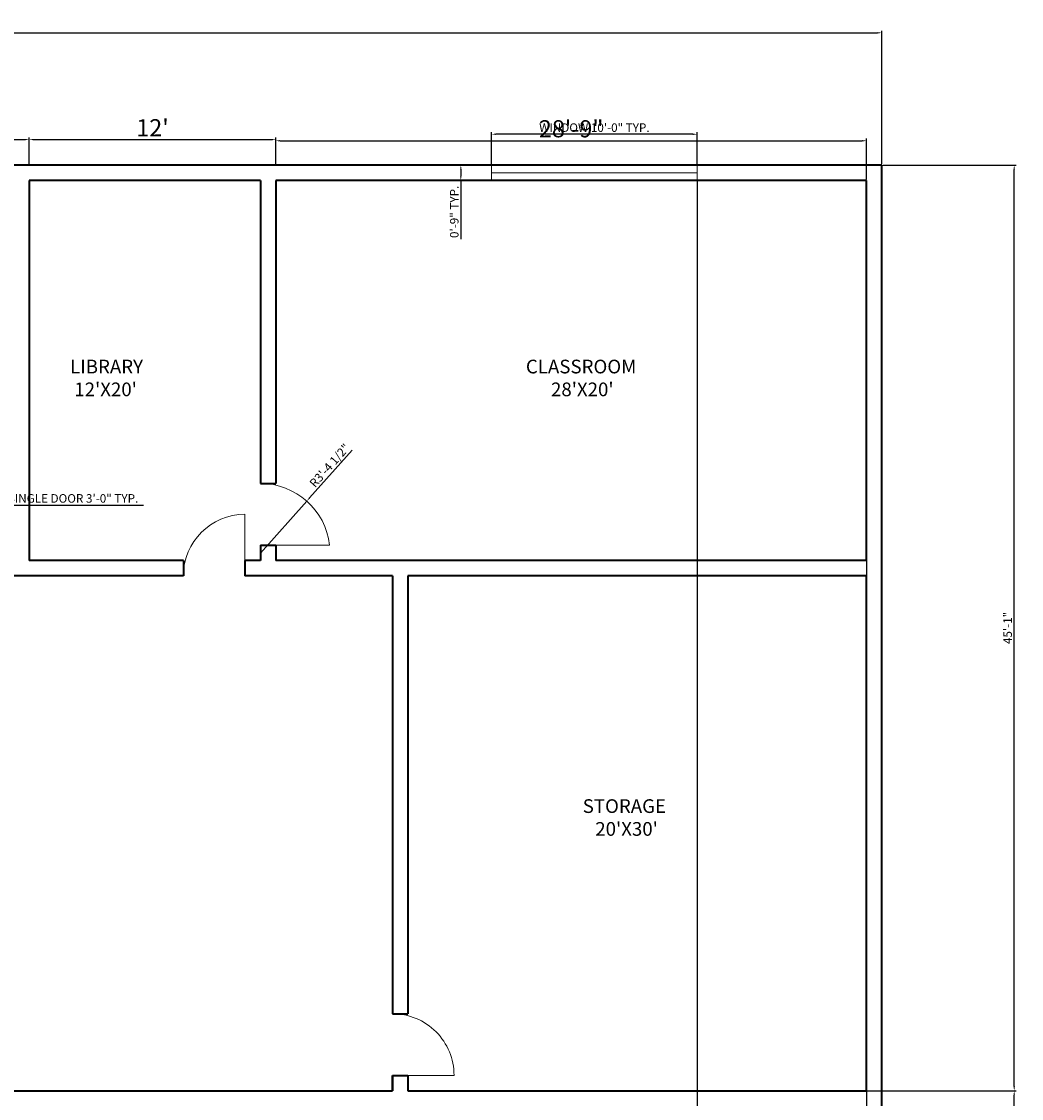
# Model space of a CAD drawing. Units: inches. Extents: x 2394 to 4066, y 1878 to 3193.
# Tile 3 of 3: x 3482 to 4066, y 2560 to 3189. Entities that reach past the tile are written whole.
import ezdxf

# ---------------------------------------------------------------- set-up
doc = ezdxf.new("R2010")
doc.units = ezdxf.units.IN
for name, color, linetype, lineweight in [('A-ANNO-DIMS', 2, 'Continuous', 13), ('A-AREA-IDEN', 7, 'Continuous', 18), ('A-DOOR', 3, 'Continuous', 18), ('A-GLAZ', 4, 'Continuous', 18), ('A-WALL', 7, 'Continuous', 35)]:
    doc.layers.add(name, color=color, linetype=linetype, lineweight=lineweight)
doc.styles.get("Standard").update_dxf_attribs({"font": 'arial.ttf'})
doc.dimstyles.new('ISO-25', dxfattribs={"dimtxt": 5, "dimasz": 2.5, "dimexe": 1.25, "dimexo": 0.625, "dimtad": 1, "dimlunit": 3, "dimtxsty": 'Standard', "dimcen": 2.5, "dimadec": 0, "dimazin": 0, "dimtfac": 1, "dimtmove": 0, "dimatfit": 3, "dimfxl": 1, "dimarcsym": 0})

# ---------------------------------------------------------------- blocks, each defined once
blk = doc.blocks.new('*D3')
at = {"layer": 'A-ANNO-DIMS', "color": 0, "lineweight": -2, "transparency": 16777216}
for p, q in [((3150.1, 3105.72), (3150.1, 3121.22)), ((3486.1, 3105.72), (3486.1, 3121.22)), ((3152.6, 3119.97), (3483.6, 3119.97))]:
    blk.add_line(p, q, dxfattribs=at)
at = {"layer": 'A-ANNO-DIMS', "color": 0, "transparency": 16777216}
for points in [[(3152.6, 3120.39), (3152.6, 3119.56), (3150.1, 3119.97)], [(3483.6, 3120.39), (3483.6, 3119.56), (3486.1, 3119.97)]]:
    blk.add_solid(points, dxfattribs=at)
at = {"layer": 'Defpoints', "color": 0, "transparency": 16777216}
for p in [(3486.1, 3119.97), (3150.1, 3105.09), (3486.1, 3105.09)]:
    blk.add_point(p, dxfattribs=at)
at = {"layer": 'A-ANNO-DIMS', "color": 0, "transparency": 16777216, "insert": (3318.1, 3125.7), "char_height": 10, "attachment_point": 5}
blk.add_mtext("28'", dxfattribs=at)
blk = doc.blocks.new('*D4')
at = {"layer": 'A-ANNO-DIMS', "color": 0, "lineweight": -2, "transparency": 16777216}
for p, q in [((3486.1, 3105.72), (3486.1, 3121.19)), ((3630.1, 3105.72), (3630.1, 3121.19)), ((3488.6, 3119.94), (3627.6, 3119.94))]:
    blk.add_line(p, q, dxfattribs=at)
at = {"layer": 'A-ANNO-DIMS', "color": 0, "transparency": 16777216}
for points in [[(3488.6, 3120.36), (3488.6, 3119.53), (3486.1, 3119.94)], [(3627.6, 3120.36), (3627.6, 3119.53), (3630.1, 3119.94)]]:
    blk.add_solid(points, dxfattribs=at)
at = {"layer": 'Defpoints', "color": 0, "transparency": 16777216}
for p in [(3630.1, 3119.94), (3486.1, 3105.09), (3630.1, 3105.09)]:
    blk.add_point(p, dxfattribs=at)
at = {"layer": 'A-ANNO-DIMS', "color": 0, "transparency": 16777216, "insert": (3558.1, 3125.59), "char_height": 10, "attachment_point": 5}
blk.add_mtext("12'", dxfattribs=at)
blk = doc.blocks.new('*D5')
at = {"layer": 'A-ANNO-DIMS', "color": 0, "lineweight": -2, "transparency": 16777216}
for p, q in [((3630.1, 3105.72), (3630.1, 3120.52)), ((3975.1, 3096.72), (3975.1, 3120.52)), ((3632.6, 3119.27), (3972.6, 3119.27))]:
    blk.add_line(p, q, dxfattribs=at)
at = {"layer": 'A-ANNO-DIMS', "color": 0, "transparency": 16777216}
for points in [[(3632.6, 3119.69), (3632.6, 3118.85), (3630.1, 3119.27)], [(3972.6, 3119.69), (3972.6, 3118.85), (3975.1, 3119.27)]]:
    blk.add_solid(points, dxfattribs=at)
at = {"layer": 'Defpoints', "color": 0, "transparency": 16777216}
for p in [(3975.1, 3119.27), (3630.1, 3105.09), (3975.1, 3096.09)]:
    blk.add_point(p, dxfattribs=at)
at = {"layer": 'A-ANNO-DIMS', "color": 0, "transparency": 16777216, "insert": (3802.6, 3125), "char_height": 10, "attachment_point": 5}
blk.add_mtext('28\'-9"', dxfattribs=at)
blk = doc.blocks.new('DOOR-SINGLE-36IN')
blk.add_line((36, 0), (36, 36))
blk.add_arc((36, 0), 36, 90, 180)
blk = doc.blocks.new('WINDOW-120IN')
for p, q in [((0, 0), (0, 9)), ((120, 0), (120, 9)), ((120, 4.5), (0, 4.5))]:
    blk.add_line(p, q)
blk = doc.blocks.new('*D15')
at = {"layer": 'A-ANNO-DIMS', "color": 0, "lineweight": -2, "transparency": 16777216}
for p, q in [((3432.1, 2901.72), (3432.1, 2907.74)), ((3434.6, 2906.49), (3465.6, 2906.49)), ((3468.1, 2901.72), (3468.1, 2907.74)), ((3468.1, 2906.49), (3552.76, 2906.49))]:
    blk.add_line(p, q, dxfattribs=at)
at = {"layer": 'A-ANNO-DIMS', "color": 0, "transparency": 16777216}
for points in [[(3434.6, 2906.91), (3434.6, 2906.08), (3432.1, 2906.49)], [(3465.6, 2906.91), (3465.6, 2906.08), (3468.1, 2906.49)]]:
    blk.add_solid(points, dxfattribs=at)
at = {"layer": 'Defpoints', "color": 0, "transparency": 16777216}
for p in [(3468.1, 2906.49), (3432.1, 2901.09), (3468.1, 2901.09)]:
    blk.add_point(p, dxfattribs=at)
at = {"layer": 'A-ANNO-DIMS', "color": 0, "transparency": 16777216, "insert": (3511.68, 2909.71), "char_height": 5, "attachment_point": 5}
blk.add_mtext('SINGLE DOOR 3\'-0" TYP.', dxfattribs=at)
blk = doc.blocks.new('*D17')
at = {"layer": 'A-ANNO-DIMS', "color": 0, "lineweight": -2, "transparency": 16777216}
for p, q in [((3756.16, 3105.72), (3756.16, 3124.34)), ((3873.66, 3123.09), (3758.66, 3123.09)), ((3876.16, 3105.72), (3876.16, 3124.34))]:
    blk.add_line(p, q, dxfattribs=at)
at = {"layer": 'A-ANNO-DIMS', "color": 0, "transparency": 16777216}
for points in [[(3758.66, 3123.51), (3758.66, 3122.68), (3756.16, 3123.09)], [(3873.66, 3123.51), (3873.66, 3122.68), (3876.16, 3123.09)]]:
    blk.add_solid(points, dxfattribs=at)
at = {"layer": 'Defpoints', "color": 0, "transparency": 16777216}
for p in [(3756.16, 3123.09), (3756.16, 3105.09), (3876.16, 3105.09)]:
    blk.add_point(p, dxfattribs=at)
at = {"layer": 'A-ANNO-DIMS', "color": 0, "transparency": 16777216, "insert": (3816.16, 3126.3), "char_height": 5, "attachment_point": 5}
blk.add_mtext('WINDOW 10\'-0" TYP.', dxfattribs=at)
blk = doc.blocks.new('*D18')
at = {"layer": 'A-ANNO-DIMS', "color": 0, "lineweight": -2, "transparency": 16777216}
for p, q in [((3755.53, 3105.09), (3736.91, 3105.09)), ((3738.16, 3102.59), (3738.16, 3098.59)), ((3755.53, 3096.09), (3736.91, 3096.09)), ((3738.16, 3096.09), (3738.16, 3061.86))]:
    blk.add_line(p, q, dxfattribs=at)
at = {"layer": 'A-ANNO-DIMS', "color": 0, "transparency": 16777216}
for points in [[(3737.74, 3102.59), (3738.57, 3102.59), (3738.16, 3105.09)], [(3737.74, 3098.59), (3738.57, 3098.59), (3738.16, 3096.09)]]:
    blk.add_solid(points, dxfattribs=at)
at = {"layer": 'Defpoints', "color": 0, "transparency": 16777216}
for p in [(3756.16, 3105.09), (3738.16, 3096.09), (3756.16, 3096.09)]:
    blk.add_point(p, dxfattribs=at)
at = {"layer": 'A-ANNO-DIMS', "color": 0, "transparency": 16777216, "insert": (3734.98, 3077.73), "char_height": 5, "attachment_point": 5, "rotation": 90}
blk.add_mtext('0\'-9" TYP.', dxfattribs=at)
blk = doc.blocks.new('*D19')
at = {"layer": 'A-ANNO-DIMS', "color": 0, "lineweight": -2, "transparency": 16777216}
for p, q in [((2478.1, 3105.72), (2478.1, 3183.59)), ((3984.1, 3105.72), (3984.1, 3183.59)), ((2480.6, 3182.34), (3981.6, 3182.34))]:
    blk.add_line(p, q, dxfattribs=at)
at = {"layer": 'A-ANNO-DIMS', "color": 0, "transparency": 16777216}
for points in [[(2480.6, 3182.76), (2480.6, 3181.93), (2478.1, 3182.34)], [(3981.6, 3182.76), (3981.6, 3181.93), (3984.1, 3182.34)]]:
    blk.add_solid(points, dxfattribs=at)
at = {"layer": 'Defpoints', "color": 0, "transparency": 16777216}
for p in [(3984.1, 3182.34), (2478.1, 3105.09), (3984.1, 3105.09)]:
    blk.add_point(p, dxfattribs=at)
at = {"layer": 'A-ANNO-DIMS', "color": 0, "transparency": 16777216, "insert": (3231.1, 3185.52), "char_height": 5, "attachment_point": 5}
blk.add_mtext('125\'-6"', dxfattribs=at)
blk = doc.blocks.new('*D27')
at = {"layer": 'A-ANNO-DIMS', "color": 0, "lineweight": -2, "transparency": 16777216}
for p, q in [((3975.72, 2564.33), (4062.6, 2564.33)), ((4061.35, 2303.14), (4061.35, 2561.83)), ((3975.72, 2300.64), (4062.6, 2300.64))]:
    blk.add_line(p, q, dxfattribs=at)
at = {"layer": 'A-ANNO-DIMS', "color": 0, "transparency": 16777216}
for points in [[(4060.93, 2561.83), (4061.76, 2561.83), (4061.35, 2564.33)], [(4060.93, 2303.14), (4061.76, 2303.14), (4061.35, 2300.64)]]:
    blk.add_solid(points, dxfattribs=at)
at = {"layer": 'Defpoints', "color": 0, "transparency": 16777216}
for p in [(3975.1, 2564.33), (4061.35, 2564.33), (3975.1, 2300.64)]:
    blk.add_point(p, dxfattribs=at)
at = {"layer": 'A-ANNO-DIMS', "color": 0, "transparency": 16777216, "insert": (4058.14, 2432.49), "char_height": 5, "attachment_point": 5, "rotation": 90}
blk.add_mtext('21\'-11 1/2"', dxfattribs=at)
blk = doc.blocks.new('*D28')
at = {"layer": 'A-ANNO-DIMS', "color": 0, "lineweight": -2, "transparency": 16777216}
for p, q in [((3984.72, 3105.09), (4062.6, 3105.09)), ((4061.35, 2566.83), (4061.35, 3102.59)), ((3975.72, 2564.33), (4062.6, 2564.33))]:
    blk.add_line(p, q, dxfattribs=at)
at = {"layer": 'A-ANNO-DIMS', "color": 0, "transparency": 16777216}
for points in [[(4060.93, 3102.59), (4061.76, 3102.59), (4061.35, 3105.09)], [(4060.93, 2566.83), (4061.76, 2566.83), (4061.35, 2564.33)]]:
    blk.add_solid(points, dxfattribs=at)
at = {"layer": 'Defpoints', "color": 0, "transparency": 16777216}
for p in [(3984.1, 3105.09), (4061.35, 3105.09), (3975.1, 2564.33)]:
    blk.add_point(p, dxfattribs=at)
at = {"layer": 'A-ANNO-DIMS', "color": 0, "transparency": 16777216, "insert": (4058.17, 2834.71), "char_height": 5, "attachment_point": 5, "rotation": 90}
blk.add_mtext('45\'-1"', dxfattribs=at)
blk = doc.blocks.new('*D33')
at = {"layer": 'A-ANNO-DIMS', "color": 0, "lineweight": -2, "transparency": 16777216}
for p, q in [((3876.16, 3095.47), (3876.16, 1880.59)), ((3975.1, 3095.47), (3975.1, 1880.59)), ((3878.66, 1881.84), (3972.6, 1881.84))]:
    blk.add_line(p, q, dxfattribs=at)
at = {"layer": 'A-ANNO-DIMS', "color": 0, "transparency": 16777216}
for points in [[(3878.66, 1882.26), (3878.66, 1881.43), (3876.16, 1881.84)], [(3972.6, 1882.26), (3972.6, 1881.43), (3975.1, 1881.84)]]:
    blk.add_solid(points, dxfattribs=at)
at = {"layer": 'Defpoints', "color": 0, "transparency": 16777216}
for p in [(3876.16, 3096.09), (3975.1, 3096.09), (3975.1, 1881.84)]:
    blk.add_point(p, dxfattribs=at)
at = {"layer": 'A-ANNO-DIMS', "color": 0, "transparency": 16777216, "insert": (3925.63, 1885.02), "char_height": 5, "attachment_point": 5}
blk.add_mtext('8\'-3"', dxfattribs=at)
blk = doc.blocks.new('*D36')
at = {"layer": 'A-ANNO-DIMS', "color": 0, "lineweight": -2, "transparency": 16777216}
for p, q in [((3674.71, 2938.6), (3649.83, 2910.66)), ((3621.1, 2878.38), (3648.17, 2908.79))]:
    blk.add_line(p, q, dxfattribs=at)
at = {"layer": 'A-ANNO-DIMS', "color": 0, "transparency": 16777216}
blk.add_solid([(3649.52, 2910.93), (3650.14, 2910.38), (3648.17, 2908.79)], dxfattribs=at)
at = {"layer": 'Defpoints', "color": 0, "transparency": 16777216}
for p in [(3648.17, 2908.79), (3621.1, 2878.38)]:
    blk.add_point(p, dxfattribs=at)
at = {"layer": 'A-ANNO-DIMS', "color": 0, "transparency": 16777216, "insert": (3662.01, 2929.17), "char_height": 5, "attachment_point": 5, "rotation": 48.32519}
blk.add_mtext('R3\'-4 1/2"', dxfattribs=at)

msp = doc.modelspace()

# ---------------------------------------------------------------- linework, layer by layer
at = {"layer": 'A-DOOR'}
for p, q in [((3621.098, 2883.092), (3657.098, 2883.092)), ((3657.098, 2883.092), (3661.539, 2883.092))]:
    msp.add_line(p, q, dxfattribs=at)
msp.add_arc((3621.098, 2878.377), 40.715, 6.650401, 90, dxfattribs=at)
at = {"layer": 'A-WALL'}
for p, q in [((3984.098, 3105.092), (2478.098, 3105.092)), ((3984.098, 1959.092), (3984.098, 3105.092)), ((3486.098, 3096.092), (3486.098, 2874.092)), ((3621.098, 3096.092), (3486.098, 3096.092)), ((3621.098, 3096.092), (3621.098, 2919.092)), ((3975.098, 3096.092), (3630.098, 3096.092)), ((3630.098, 3096.092), (3630.098, 2919.092)), ((3975.098, 2874.092), (3975.098, 3096.092)), ((3621.098, 2919.092), (3630.098, 2919.092)), ((3621.098, 2883.092), (3630.098, 2883.092)), ((3621.098, 2883.092), (3621.098, 2874.092)), ((3630.098, 2883.092), (3630.098, 2874.092)), ((3576.098, 2874.092), (3486.098, 2874.092)), ((3576.098, 2874.092), (3576.098, 2865.092)), ((3621.098, 2874.092), (3612.098, 2874.092)), ((3612.098, 2874.092), (3612.098, 2865.092)), ((3975.098, 2874.092), (3630.098, 2874.092)), ((3576.098, 2865.092), (3468.098, 2865.092)), ((3698.204, 2865.092), (3612.098, 2865.092)), ((3698.204, 2865.092), (3698.204, 2609.327)), ((3975.098, 2865.092), (3707.204, 2865.092)), ((3707.204, 2865.092), (3707.204, 2609.327)), ((3975.098, 2564.327), (3975.098, 2865.092)), ((3698.204, 2609.327), (3707.204, 2609.327)), ((3698.204, 2564.327), (3698.204, 2573.327)), ((3698.204, 2573.327), (3707.204, 2573.327)), ((3698.204, 2573.327), (3698.204, 2564.327)), ((3707.204, 2573.327), (3707.204, 2564.327)), ((2986.598, 2564.327), (3698.204, 2564.327)), ((3707.204, 2564.327), (3975.098, 2564.327))]:
    msp.add_line(p, q, dxfattribs=at)

# ---------------------------------------------------------------- block references
at = {"layer": 'A-DOOR'}
msp.add_blockref('DOOR-SINGLE-36IN', (3576.098, 2865.092), dxfattribs=at)
at = {"layer": 'A-DOOR', "rotation": 270.0000000000003}
msp.add_blockref('DOOR-SINGLE-36IN', (3698.204, 2609.327), dxfattribs=at)
at = {"layer": 'A-GLAZ', "rotation": 180}
msp.add_blockref('WINDOW-120IN', (3876.156, 3105.092), dxfattribs=at)

# ---------------------------------------------------------------- texts
at = {"layer": 'A-AREA-IDEN', "char_height": 8, "attachment_point": 1}
for s, insert in [("LIBRARY\\P 12'X20'", (3509.97, 2991.385)), ("CLASSROOM\\P      28'X20'", (3776.158, 2991.385)), ("STORAGE\\P   20'X30'", (3809.353, 2734.617))]:
    msp.add_mtext_dynamic_manual_height_columns(s, width=162.41234, gutter_width=12.5, heights=[0], dxfattribs=dict(at, insert=insert))

# ---------------------------------------------------------------- dimensions: what is measured, and where the dimension line sits
at = {"layer": 'A-ANNO-DIMS'}
for base, p1, p2, override, picture, middle in [((3984.098, 3182.342), (2478.098, 3105.092), (3984.098, 3105.092), {"dimdec": 1, "dimlfac": 1, "dimrnd": 0, "dimzin": 1, "dimdsep": 46, "dimlunit": 4, "dimfrac": 2}, '*D19', (3231.098, 3185.52)), ((3486.098, 3119.972), (3150.098, 3105.092), (3486.098, 3105.092), {"dimtxt": 10, "dimclrd": 0, "dimclre": 0, "dimclrt": 0}, '*D3', (3318.098, 3125.703)), ((3630.098, 3119.943), (3486.098, 3105.092), (3630.098, 3105.092), {"dimtxt": 10, "dimclrd": 0, "dimclre": 0, "dimclrt": 0}, '*D4', (3558.098, 3125.589)), ((3975.098, 3119.27), (3630.098, 3105.092), (3975.098, 3096.092), {"dimtxt": 10, "dimclrd": 0, "dimclre": 0, "dimclrt": 0}, '*D5', (3802.598, 3125)), ((3975.098, 1881.842), (3876.157, 3096.092), (3975.098, 3096.092), {"dimdec": 1, "dimlfac": 1, "dimrnd": 0, "dimzin": 1, "dimdsep": 46, "dimlunit": 4, "dimfrac": 2}, '*D33', (3925.627, 1885.022))]:
    dim = msp.add_linear_dim(base=base, p1=p1, p2=p2, dimstyle='ISO-25', override=override, dxfattribs=at)
    dim.commit()
    dim.dimension.update_dxf_attribs({"geometry": picture, "text_midpoint": middle})
for base, p1, p2, angle, text, picture, middle in [((3756.157, 3123.092), (3876.157, 3105.092), (3756.157, 3105.092), 180, 'WINDOW <> TYP.', '*D17', (3816.157, 3126.304)), ((3738.157, 3096.092), (3756.157, 3105.092), (3756.157, 3096.092), 270, '<> TYP.', '*D18', (3734.979, 3077.728))]:
    dim = msp.add_linear_dim(base=base, p1=p1, p2=p2, angle=angle, text=text, dimstyle='ISO-25', override={"dimdec": 1, "dimlfac": 1, "dimrnd": 0, "dimzin": 1, "dimdsep": 46, "dimlunit": 4, "dimfrac": 2}, dxfattribs=at)
    dim.commit()
    dim.dimension.update_dxf_attribs({"geometry": picture, "text_midpoint": middle})
for base, p1, p2, picture, middle in [((4061.348, 3105.092), (3975.098, 2564.327), (3984.098, 3105.092), '*D28', (4058.17, 2834.71)), ((4061.348, 2564.327), (3975.098, 2300.645), (3975.098, 2564.327), '*D27', (4058.137, 2432.486))]:
    dim = msp.add_linear_dim(base=base, p1=p1, p2=p2, angle=90, dimstyle='ISO-25', override={"dimdec": 1, "dimlfac": 1, "dimrnd": 0, "dimzin": 1, "dimdsep": 46, "dimlunit": 4, "dimfrac": 2}, dxfattribs=at)
    dim.commit()
    dim.dimension.update_dxf_attribs({"geometry": picture, "text_midpoint": middle})
dim = msp.add_radius_dim(center=(3621.098, 2878.377), mpoint=(3648.169, 2908.788), dimstyle='ISO-25', override={"dimdec": 1, "dimlfac": 1, "dimrnd": 0, "dimzin": 1, "dimdsep": 46, "dimlunit": 4, "dimfrac": 2}, dxfattribs=at)
dim.commit()
dim.dimension.update_dxf_attribs({"geometry": '*D36', "text_midpoint": (3664.412, 2927.035), "dimtype": 164})
dim = msp.add_linear_dim(base=(3468.098, 2906.492), p1=(3432.098, 2901.092), p2=(3468.098, 2901.092), text='SINGLE DOOR <> TYP.', dimstyle='ISO-25', override={"dimdec": 1, "dimlfac": 1, "dimrnd": 0, "dimzin": 1, "dimdsep": 46, "dimlunit": 4, "dimfrac": 2}, dxfattribs=at)
dim.commit()
dim.dimension.update_dxf_attribs({"geometry": '*D15', "text_midpoint": (3511.678, 2909.706)})

doc.saveas('drawing.dxf')
